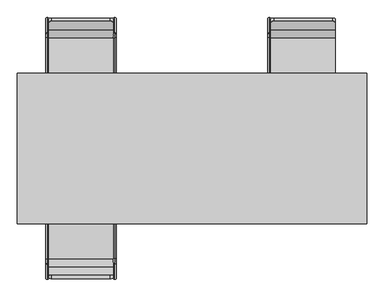
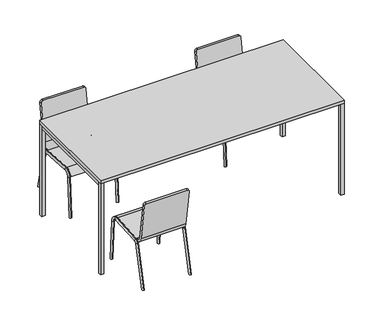
"""IFC4 building model written with IfcOpenShell, lengths in millimetres: furniture geometry."""

from ifc_helpers import new_model, si_unit, point, frame, origin, origin_with_axes, place, context, project, spatial, polyline, circle_curve, ellipse_curve, trimmed, outline, extrude, source, transform, mapped, element, save
from ifc_brep_helpers import plane_surface, cylinder_surface, revolved_surface, advanced_brep


def furniture_b3e58817(model_context):
    return source(origin(), model_context, "Body", "SolidModel", [
        advanced_brep(
        [(10.8556283, 323.0385228, 0.0), (0.8556283, 313.0554101, 0.5809138), (-9.1443717, 323.0385228, 0.0), (0.8556283, 709.1722272, 383.1163586), (0.8556283, 728.5781417, 387.9547965), (0.8556283, 825.3061363, 0.0), (0.8556283, 804.6938637, 0.0), (0.8556283, 333.0554387, 0.0), (0.8556283, 696.6509897, 414.4284246), (0.8556283, 695.489162, 394.4621992), (0.8556283, 397.0871192, 411.8261096), (0.8556283, 398.2489468, 431.792335), (0.8556283, 354.8310131, 374.2173141), (0.8556283, 334.8647877, 375.3791418)],
        [
            (0, 1, circle_curve(frame((0.8556283, 323.0385228, 0.0), z_axis=(0.0, -0.058091383027392335, -0.9983112697039761), x_axis=(0.0, -0.9983112697039761, 0.058091383027392335)), 10.0)),
            (1, 2, circle_curve(frame((0.8556283, 323.0385228, 0.0), z_axis=(0.0, -0.058091383027392335, -0.9983112697039761), x_axis=(0.0, -0.9983112697039761, 0.058091383027392335)), 10.0)),
            (2, 0),
            (3, 4, circle_curve(frame((0.8556283, 718.8751844, 385.5355776), z_axis=(0.0, 0.24192189559966623, -0.9702957262759968), x_axis=(0.0, 0.9702957262759968, 0.24192189559966623)), 10.0)),
            (4, 5),
            (5, 6, ellipse_curve(frame((0.8556283, 815.0, 0.0), z_axis=(0.0, 0.0, 1.0), x_axis=(0.0, 1.0, 0.0)), 10.3061363, 10.0)),
            (6, 3),
            (4, 3, circle_curve(frame((0.8556283, 718.8751844, 385.5355776), z_axis=(0.0, 0.24192189559966623, -0.9702957262759968), x_axis=(0.0, 0.9702957262759968, 0.24192189559966623)), 10.0)),
            (6, 5, ellipse_curve(frame((0.8556283, 815.0, 0.0), z_axis=(0.0, 0.0, 1.0), x_axis=(0.0, 1.0, 0.0)), 10.3061363, 10.0)),
            (2, 7, ellipse_curve(frame((0.8556283, 323.0385228, 0.0), z_axis=(0.0, 0.0, -1.0), x_axis=(0.0, 1.0, 0.0)), 10.0169159, 10.0)),
            (7, 0, ellipse_curve(frame((0.8556283, 323.0385228, 0.0), z_axis=(0.0, 0.0, -1.0), x_axis=(0.0, 1.0, 0.0)), 10.0169159, 10.0)),
            (8, 9, circle_curve(frame((0.8556283, 696.0700758, 404.4453119), z_axis=(0.0, -0.9983112697039764, 0.058091383027386895), x_axis=(0.0, 0.058091383027386895, 0.9983112697039764)), 10.0)),
            (9, 10),
            (10, 11, circle_curve(frame((0.8556283, 397.668033, 421.8092223), z_axis=(0.0, 0.9983112697039764, -0.058091383027386895), x_axis=(0.0, 0.058091383027386895, 0.9983112697039764)), 10.0)),
            (11, 8),
            (9, 8, circle_curve(frame((0.8556283, 696.0700758, 404.4453119), z_axis=(0.0, -0.9983112697039764, 0.058091383027386895), x_axis=(0.0, 0.058091383027386895, 0.9983112697039764)), 10.0)),
            (11, 10, circle_curve(frame((0.8556283, 397.668033, 421.8092223), z_axis=(0.0, 0.9983112697039764, -0.058091383027386895), x_axis=(0.0, 0.058091383027386895, 0.9983112697039764)), 10.0)),
            (10, 12, circle_curve(frame((0.8556283, 394.7634639, 371.8936588), z_axis=(1.0, 0.0, 0.0), x_axis=(0.0, 0.05809138302738633, 0.9983112697039764)), 40.0)),
            (12, 13, circle_curve(frame((0.8556283, 344.8479004, 374.7982279), z_axis=(0.0, 0.058091383027391474, 0.9983112697039761), x_axis=(0.0, -0.9983112697039761, 0.058091383027391474)), 10.0)),
            (13, 11, circle_curve(frame((0.8556283, 394.7634639, 371.8936588), z_axis=(-1.0, 0.0, 0.0), x_axis=(0.0, 0.05809138302738633, 0.9983112697039764)), 60.0)),
            (13, 12, circle_curve(frame((0.8556283, 344.8479004, 374.7982279), z_axis=(0.0, 0.05809138302739081, 0.9983112697039762), x_axis=(0.0, -0.9983112697039762, 0.05809138302739081)), 10.0)),
            (12, 7),
            (1, 13),
            (3, 9, circle_curve(frame((0.8556283, 694.6177913, 379.4875302), z_axis=(1.0, 0.0, 0.0), x_axis=(0.0, 0.9702957262759969, 0.2419218955996659)), 15.0)),
            (8, 4, circle_curve(frame((0.8556283, 694.6177913, 379.4875302), z_axis=(-1.0, 0.0, 0.0), x_axis=(0.0, 0.9702957262759969, 0.2419218955996659)), 35.0)),
        ],
        [
            plane_surface(frame((20.8556283, 323.0385228, 0.0), z_axis=(0.0, -0.058091383027392335, -0.9983112697039761), x_axis=(-1.0, 0.0, 0.0))),
            cylinder_surface(frame((0.8556283, 817.6101503, -10.4687411), z_axis=(0.0, 0.24192189559966623, -0.9702957262759968), x_axis=(0.0, 0.9702957262759968, 0.24192189559966623)), 10.0),
            plane_surface(frame((463.435329, 850.4463822, 0.0), z_axis=(0.0, 0.0, -1.0), x_axis=(-1.0, 0.0, 0.0))),
            cylinder_surface(frame((0.8556283, 696.0700758, 404.4453119), z_axis=(0.0, 0.9983112697039764, -0.058091383027386895), x_axis=(0.0, 0.058091383027386895, 0.9983112697039764)), 10.0),
            revolved_surface(trimmed(ellipse_curve(frame((0.8556283, 397.668033, 421.8092223), z_axis=(0.0, 0.9983112697039764, -0.05809138302738631), x_axis=(0.0, 0.05809138302738631, 0.9983112697039764)), 10.0, 10.0), [point((0.8556283, 397.0871192, 411.8261096))], [point((0.8556283, 398.2489468, 431.792335))], True, "CARTESIAN"), (20.8556283, 394.7634639, 371.8936588), (1.0, 0.0, 0.0)),
            revolved_surface(trimmed(ellipse_curve(frame((0.8556283, 397.668033, 421.8092223), z_axis=(0.0, 0.9983112697039764, -0.05809138302738631), x_axis=(0.0, 0.05809138302738631, 0.9983112697039764)), 10.0, 10.0), [point((0.8556283, 398.2489468, 431.792335))], [point((0.8556283, 397.0871192, 411.8261096))], True, "CARTESIAN"), (20.8556283, 394.7634639, 371.8936588), (1.0, 0.0, 0.0)),
            cylinder_surface(frame((0.8556283, 344.8479004, 374.7982279), z_axis=(0.0, 0.058091383027392335, 0.9983112697039761), x_axis=(0.0, -0.9983112697039761, 0.058091383027392335)), 10.0),
            revolved_surface(trimmed(ellipse_curve(frame((0.8556283, 718.8751844, 385.5355776), z_axis=(0.0, 0.2419218955996659, -0.9702957262759969), x_axis=(0.0, 0.9702957262759969, 0.2419218955996659)), 10.0, 10.0), [point((0.8556283, 709.1722272, 383.1163586))], [point((0.8556283, 728.5781417, 387.9547965))], True, "CARTESIAN"), (20.8556283, 694.6177913, 379.4875302), (1.0, 0.0, 0.0)),
            revolved_surface(trimmed(ellipse_curve(frame((0.8556283, 718.8751844, 385.5355776), z_axis=(0.0, 0.2419218955996659, -0.9702957262759969), x_axis=(0.0, 0.9702957262759969, 0.2419218955996659)), 10.0, 10.0), [point((0.8556283, 728.5781417, 387.9547965))], [point((0.8556283, 709.1722272, 383.1163586))], True, "CARTESIAN"), (20.8556283, 694.6177913, 379.4875302), (1.0, 0.0, 0.0)),
        ],
        [
            (0, [[1, 2, 3]]),
            (1, [[4, 5, 6, 7]]),
            (1, [[8, -7, 9, -5]]),
            (2, [[-3, 10, 11]]),
            (2, [[-6, -9]]),
            (3, [[12, 13, 14, 15]]),
            (3, [[16, -15, 17, -13]]),
            (4, [[-14, 18, 19, 20]]),
            (5, [[-17, -20, 21, -18]]),
            (6, [[-19, 22, -10, -2, 23]]),
            (6, [[-21, -23, -1, -11, -22]]),
            (7, [[-4, 24, -12, 25]]),
            (8, [[-8, -25, -16, -24]]),
        ],
    ),
        advanced_brep(
        [(415.935329, 694.2901891, 414.5657988), (415.935329, 398.2489468, 431.792335), (415.935329, 334.8647877, 375.3791418), (415.935329, 354.8310131, 374.2173141), (415.935329, 397.0871192, 411.8261096), (415.935329, 693.1283614, 394.5995734), (415.935329, 766.4258686, 454.1347035), (415.935329, 817.282073, 794.4215124), (415.935329, 797.5017557, 797.3777006), (415.935329, 746.6455514, 457.0908917), (10.935329, 694.2901891, 414.5657988), (10.935329, 746.6455514, 457.0908917), (10.935329, 797.5017557, 797.3777006), (10.935329, 817.282073, 794.4215124), (10.935329, 766.4258686, 454.1347035), (10.935329, 693.1283614, 394.5995734), (10.935329, 397.0871192, 411.8261096), (10.935329, 354.8310131, 374.2173141), (10.935329, 334.8647877, 375.3791418), (10.935329, 398.2489468, 431.792335), (30.935329, 820.2382612, 814.2018297), (395.935329, 820.2382612, 814.2018297), (30.935329, 800.4579439, 817.1580179), (395.935329, 800.4579439, 817.1580179)],
        [
            (0, 1),
            (1, 2, circle_curve(frame((415.935329, 394.7634639, 371.8936588), z_axis=(1.0, 0.0, 0.0), x_axis=(0.0, 1.0, 0.0)), 60.0)),
            (2, 3),
            (3, 4, circle_curve(frame((415.935329, 394.7634639, 371.8936588), z_axis=(-1.0, 0.0, 0.0), x_axis=(0.0, 1.0, 0.0)), 40.0)),
            (4, 5),
            (5, 6, circle_curve(frame((415.935329, 697.1947582, 464.4813623), z_axis=(1.0, 0.0, 0.0), x_axis=(0.0, 1.0, 0.0)), 70.0)),
            (6, 7),
            (7, 8),
            (8, 9),
            (9, 0, circle_curve(frame((415.935329, 697.1947582, 464.4813623), z_axis=(-1.0, 0.0, 0.0), x_axis=(0.0, 1.0, 0.0)), 50.0)),
            (10, 11, circle_curve(frame((10.935329, 697.1947582, 464.4813623), z_axis=(1.0, 0.0, 0.0), x_axis=(0.0, 1.0, 0.0)), 50.0)),
            (11, 12),
            (12, 13),
            (13, 14),
            (14, 15, circle_curve(frame((10.935329, 697.1947582, 464.4813623), z_axis=(-1.0, 0.0, 0.0), x_axis=(0.0, 1.0, 0.0)), 70.0)),
            (15, 16),
            (16, 17, circle_curve(frame((10.935329, 394.7634639, 371.8936588), z_axis=(1.0, 0.0, 0.0), x_axis=(0.0, 1.0, 0.0)), 40.0)),
            (17, 18),
            (18, 19, circle_curve(frame((10.935329, 394.7634639, 371.8936588), z_axis=(-1.0, 0.0, 0.0), x_axis=(0.0, 1.0, 0.0)), 60.0)),
            (19, 10),
            (0, 10),
            (19, 1),
            (18, 2),
            (17, 3),
            (16, 4),
            (15, 5),
            (14, 6),
            (13, 20, circle_curve(frame((30.935329, 817.282073, 794.4215124), z_axis=(0.0, 0.9890158633619166, -0.14780941112961252), x_axis=(1.0, 0.0, 0.0)), 20.0)),
            (20, 21),
            (21, 7, circle_curve(frame((395.935329, 817.282073, 794.4215124), z_axis=(0.0, 0.9890158633619166, -0.14780941112961252), x_axis=(-1.0, 0.0, 0.0)), 20.0)),
            (20, 22),
            (22, 23),
            (23, 21),
            (11, 9),
            (8, 23, circle_curve(frame((395.935329, 797.5017557, 797.3777006), z_axis=(0.0, -0.9890158633619166, 0.14780941112961252), x_axis=(-1.0, 0.0, 0.0)), 20.0)),
            (22, 12, circle_curve(frame((30.935329, 797.5017557, 797.3777006), z_axis=(0.0, -0.9890158633619166, 0.14780941112961252), x_axis=(1.0, 0.0, 0.0)), 20.0)),
        ],
        [
            plane_surface(frame((415.935329, 400.4940122, 431.6616954), z_axis=(1.0000000000000002, 0.0, 0.0), x_axis=(0.0, -0.9983112697039764, 0.05809138302738736))),
            plane_surface(frame((10.935329, 400.4940122, 431.6616954), z_axis=(-1.0000000000000002, 0.0, 0.0), x_axis=(0.0, 0.9983112697039764, -0.05809138302738736))),
            plane_surface(frame((415.935329, 694.2901891, 414.5657988), z_axis=(0.0, 0.05809138302738736, 0.9983112697039764), x_axis=(-1.0, 0.0, 0.0))),
            cylinder_surface(frame((10.935329, 394.7634639, 371.8936588), z_axis=(1.0, 0.0, 0.0), x_axis=(0.0, 1.0, 0.0)), 60.0),
            plane_surface(frame((415.935329, 334.8647877, 375.3791418), z_axis=(0.0, -0.058091383027390926, -0.9983112697039762), x_axis=(-1.0, 0.0, 0.0))),
            revolved_surface(polyline([(10.935329, 434.7634639, 371.8936588), (415.935329, 434.7634639, 371.8936588)]), (10.935329, 394.7634639, 371.8936588), (-1.0, 0.0, 0.0)),
            plane_surface(frame((415.935329, 397.0871192, 411.8261096), z_axis=(0.0, -0.05809138302738756, -0.9983112697039763), x_axis=(-1.0, 0.0, 0.0))),
            cylinder_surface(frame((10.935329, 697.1947582, 464.4813623), z_axis=(1.0, 0.0, 0.0), x_axis=(0.0, 1.0, 0.0)), 70.0),
            plane_surface(frame((415.935329, 766.4258686, 454.1347035), z_axis=(0.0, 0.9890158633619166, -0.1478094111296125), x_axis=(-1.0, 0.0, 0.0))),
            plane_surface(frame((415.935329, 820.2382612, 814.2018297), z_axis=(0.0, 0.14780941112961524, 0.9890158633619162), x_axis=(-1.0, 0.0, 0.0))),
            plane_surface(frame((415.935329, 800.4579439, 817.1580179), z_axis=(0.0, -0.9890158633619166, 0.14780941112961254), x_axis=(-1.0, 0.0, 0.0))),
            revolved_surface(polyline([(10.935329, 747.1947582, 464.4813623), (415.935329, 747.1947582, 464.4813623)]), (10.935329, 697.1947582, 464.4813623), (-1.0, 0.0, 0.0)),
            cylinder_surface(frame((30.935329, 797.5017557, 797.3777006), z_axis=(0.0, -0.9890158633619166, 0.14780941112961252), x_axis=(1.0, 0.0, 0.0)), 20.0),
            cylinder_surface(frame((395.935329, 797.5017557, 797.3777006), z_axis=(0.0, -0.9890158633619166, 0.14780941112961252), x_axis=(-1.0, 0.0, 0.0)), 20.0),
        ],
        [
            (0, [[1, 2, 3, 4, 5, 6, 7, 8, 9, 10]]),
            (1, [[11, 12, 13, 14, 15, 16, 17, 18, 19, 20]]),
            (2, [[-1, 21, -20, 22]]),
            (3, [[-2, -22, -19, 23]]),
            (4, [[-3, -23, -18, 24]]),
            (5, [[-4, -24, -17, 25]]),
            (6, [[-5, -25, -16, 26]]),
            (7, [[-6, -26, -15, 27]]),
            (8, [[-27, -14, 28, 29, 30, -7]]),
            (9, [[-29, 31, 32, 33]]),
            (10, [[34, -9, 35, -32, 36, -12]]),
            (11, [[-10, -34, -11, -21]]),
            (12, [[-13, -36, -31, -28]]),
            (13, [[-8, -30, -33, -35]]),
        ],
    ),
        advanced_brep(
        [(-973.9849702, -804.6938637, 0.0), (-973.9849702, -825.3061363, 0.0), (-963.9849702, -323.0385228, 0.0), (-973.9849702, -333.0554387, 0.0), (-983.9849702, -323.0385228, 0.0), (-973.9849702, -709.1722272, 383.1163586), (-973.9849702, -728.5781417, 387.9547965), (-973.9849702, -696.6509897, 414.4284246), (-973.9849702, -695.489162, 394.4621992), (-973.9849702, -398.2489468, 431.792335), (-973.9849702, -397.0871192, 411.8261096), (-973.9849702, -334.8647877, 375.3791418), (-973.9849702, -354.8310131, 374.2173141), (-973.9849702, -313.0554101, 0.5809138)],
        [
            (0, 1, ellipse_curve(frame((-973.9849702, -815.0, 0.0), z_axis=(0.0, 0.0, -1.0), x_axis=(0.0, -1.0, 0.0)), 10.3061363, 10.0)),
            (1, 0, ellipse_curve(frame((-973.9849702, -815.0, 0.0), z_axis=(0.0, 0.0, -1.0), x_axis=(0.0, -1.0, 0.0)), 10.3061363, 10.0)),
            (2, 3, ellipse_curve(frame((-973.9849702, -323.0385228, 0.0), z_axis=(0.0, 0.0, -1.0), x_axis=(0.0, -1.0, 0.0)), 10.0169159, 10.0)),
            (3, 4, ellipse_curve(frame((-973.9849702, -323.0385228, 0.0), z_axis=(0.0, 0.0, -1.0), x_axis=(0.0, -1.0, 0.0)), 10.0169159, 10.0)),
            (4, 2),
            (5, 0),
            (1, 6),
            (6, 5, circle_curve(frame((-973.9849702, -718.8751844, 385.5355776), z_axis=(0.0, -0.24192189559966623, -0.9702957262759968), x_axis=(0.0, -0.9702957262759968, 0.24192189559966623)), 10.0)),
            (5, 6, circle_curve(frame((-973.9849702, -718.8751844, 385.5355776), z_axis=(0.0, -0.24192189559966623, -0.9702957262759968), x_axis=(0.0, -0.9702957262759968, 0.24192189559966623)), 10.0)),
            (6, 7, circle_curve(frame((-973.9849702, -694.6177913, 379.4875302), z_axis=(-1.0, 0.0, 0.0), x_axis=(0.0, -0.9702957262759969, 0.2419218955996659)), 35.0)),
            (7, 8, circle_curve(frame((-973.9849702, -696.0700758, 404.4453119), z_axis=(0.0, -0.9983112697039765, -0.05809138302738456), x_axis=(0.0, -0.05809138302738456, 0.9983112697039765)), 10.0)),
            (8, 5, circle_curve(frame((-973.9849702, -694.6177913, 379.4875302), z_axis=(1.0, 0.0, 0.0), x_axis=(0.0, -0.9702957262759969, 0.2419218955996659)), 15.0)),
            (8, 7, circle_curve(frame((-973.9849702, -696.0700758, 404.4453119), z_axis=(0.0, -0.998311269703977, -0.05809138302737549), x_axis=(0.0, -0.05809138302737549, 0.998311269703977)), 10.0)),
            (7, 9),
            (9, 10, circle_curve(frame((-973.9849702, -397.668033, 421.8092223), z_axis=(0.0, -0.9983112697039764, -0.058091383027386895), x_axis=(0.0, -0.058091383027386895, 0.9983112697039764)), 10.0)),
            (10, 8),
            (10, 9, circle_curve(frame((-973.9849702, -397.668033, 421.8092223), z_axis=(0.0, -0.9983112697039764, -0.058091383027386895), x_axis=(0.0, -0.058091383027386895, 0.9983112697039764)), 10.0)),
            (9, 11, circle_curve(frame((-973.9849702, -394.7634639, 371.8936588), z_axis=(-1.0, 0.0, 0.0), x_axis=(0.0, -0.05809138302738633, 0.9983112697039764)), 60.0)),
            (11, 12, circle_curve(frame((-973.9849702, -344.8479004, 374.7982279), z_axis=(0.0, -0.05809138302739081, 0.9983112697039762), x_axis=(0.0, 0.9983112697039762, 0.05809138302739081)), 10.0)),
            (12, 10, circle_curve(frame((-973.9849702, -394.7634639, 371.8936588), z_axis=(1.0, 0.0, 0.0), x_axis=(0.0, -0.05809138302738633, 0.9983112697039764)), 40.0)),
            (12, 11, circle_curve(frame((-973.9849702, -344.8479004, 374.7982279), z_axis=(0.0, -0.05809138302739125, 0.9983112697039761), x_axis=(0.0, 0.9983112697039761, 0.05809138302739125)), 10.0)),
            (4, 13, circle_curve(frame((-973.9849702, -323.0385228, 0.0), z_axis=(0.0, 0.058091383027392335, -0.9983112697039761), x_axis=(0.0, 0.9983112697039761, 0.058091383027392335)), 10.0)),
            (13, 2, circle_curve(frame((-973.9849702, -323.0385228, 0.0), z_axis=(0.0, 0.058091383027392335, -0.9983112697039761), x_axis=(0.0, 0.9983112697039761, 0.058091383027392335)), 10.0)),
            (11, 13),
            (3, 12),
        ],
        [
            plane_surface(frame((-936.564671, -850.4463822, 0.0), z_axis=(0.0, 0.0, -1.0), x_axis=(-1.0, 0.0, 0.0))),
            cylinder_surface(frame((-973.9849702, -817.6101503, -10.4687411), z_axis=(0.0, -0.24192189559966623, -0.9702957262759968), x_axis=(0.0, -0.9702957262759968, 0.24192189559966623)), 10.0),
            revolved_surface(trimmed(ellipse_curve(frame((-973.9849702, -718.8751844, 385.5355776), z_axis=(0.0, 0.2419218955996659, 0.9702957262759969), x_axis=(0.0, -0.9702957262759969, 0.2419218955996659)), 10.0, 10.0), [point((-973.9849702, -709.1722272, 383.1163586))], [point((-973.9849702, -728.5781417, 387.9547965))], True, "CARTESIAN"), (-993.9849702, -694.6177913, 379.4875302), (1.0, 0.0, 0.0)),
            revolved_surface(trimmed(ellipse_curve(frame((-973.9849702, -718.8751844, 385.5355776), z_axis=(0.0, 0.2419218955996659, 0.9702957262759969), x_axis=(0.0, -0.9702957262759969, 0.2419218955996659)), 10.0, 10.0), [point((-973.9849702, -728.5781417, 387.9547965))], [point((-973.9849702, -709.1722272, 383.1163586))], True, "CARTESIAN"), (-993.9849702, -694.6177913, 379.4875302), (1.0, 0.0, 0.0)),
            cylinder_surface(frame((-973.9849702, -696.0700758, 404.4453119), z_axis=(0.0, -0.9983112697039764, -0.058091383027386895), x_axis=(0.0, -0.058091383027386895, 0.9983112697039764)), 10.0),
            revolved_surface(trimmed(ellipse_curve(frame((-973.9849702, -397.668033, 421.8092223), z_axis=(0.0, 0.9983112697039764, 0.05809138302738631), x_axis=(0.0, -0.05809138302738631, 0.9983112697039764)), 10.0, 10.0), [point((-973.9849702, -397.0871192, 411.8261096))], [point((-973.9849702, -398.2489468, 431.792335))], True, "CARTESIAN"), (-993.9849702, -394.7634639, 371.8936588), (1.0, 0.0, 0.0)),
            revolved_surface(trimmed(ellipse_curve(frame((-973.9849702, -397.668033, 421.8092223), z_axis=(0.0, 0.9983112697039764, 0.05809138302738631), x_axis=(0.0, -0.05809138302738631, 0.9983112697039764)), 10.0, 10.0), [point((-973.9849702, -398.2489468, 431.792335))], [point((-973.9849702, -397.0871192, 411.8261096))], True, "CARTESIAN"), (-993.9849702, -394.7634639, 371.8936588), (1.0, 0.0, 0.0)),
            plane_surface(frame((-993.9849702, -323.0385228, 0.0), z_axis=(0.0, 0.058091383027392335, -0.9983112697039761), x_axis=(1.0, 0.0, 0.0))),
            cylinder_surface(frame((-973.9849702, -344.8479004, 374.7982279), z_axis=(0.0, -0.058091383027392335, 0.9983112697039761), x_axis=(0.0, 0.9983112697039761, 0.058091383027392335)), 10.0),
        ],
        [
            (0, [[1, 2]]),
            (0, [[3, 4, 5]]),
            (1, [[6, -2, 7, 8]]),
            (1, [[-7, -1, -6, 9]]),
            (2, [[10, 11, 12, -8]]),
            (3, [[-12, 13, -10, -9]]),
            (4, [[14, 15, 16, -11]]),
            (4, [[-16, 17, -14, -13]]),
            (5, [[18, 19, 20, -15]]),
            (6, [[-20, 21, -18, -17]]),
            (7, [[-5, 22, 23]]),
            (8, [[24, -22, -4, 25, -19]]),
            (8, [[-25, -3, -23, -24, -21]]),
        ],
    ),
        advanced_brep(
        [(-1389.1443717, -323.0385228, 0.0), (-1409.1443717, -323.0385228, 0.0), (-1399.1443717, -313.0554101, 0.5809138), (-1399.1443717, -709.1722272, 383.1163586), (-1399.1443717, -804.6938637, 0.0), (-1399.1443717, -825.3061363, 0.0), (-1399.1443717, -728.5781417, 387.9547965), (-1399.1443717, -333.0554387, 0.0), (-1399.1443717, -696.6509897, 414.4284246), (-1399.1443717, -398.2489468, 431.792335), (-1399.1443717, -397.0871192, 411.8261096), (-1399.1443717, -695.489162, 394.4621992), (-1399.1443717, -334.8647877, 375.3791418), (-1399.1443717, -354.8310131, 374.2173141)],
        [
            (0, 1),
            (1, 2, circle_curve(frame((-1399.1443717, -323.0385228, 0.0), z_axis=(0.0, 0.058091383027392335, -0.9983112697039761), x_axis=(0.0, 0.9983112697039761, 0.058091383027392335)), 10.0)),
            (2, 0, circle_curve(frame((-1399.1443717, -323.0385228, 0.0), z_axis=(0.0, 0.058091383027392335, -0.9983112697039761), x_axis=(0.0, 0.9983112697039761, 0.058091383027392335)), 10.0)),
            (3, 4),
            (4, 5, ellipse_curve(frame((-1399.1443717, -815.0, 0.0), z_axis=(0.0, 0.0, 1.0), x_axis=(0.0, -1.0, 0.0)), 10.3061363, 10.0)),
            (5, 6),
            (6, 3, circle_curve(frame((-1399.1443717, -718.8751844, 385.5355776), z_axis=(0.0, -0.24192189559966623, -0.9702957262759968), x_axis=(0.0, -0.9702957262759968, 0.24192189559966623)), 10.0)),
            (5, 4, ellipse_curve(frame((-1399.1443717, -815.0, 0.0), z_axis=(0.0, 0.0, 1.0), x_axis=(0.0, -1.0, 0.0)), 10.3061363, 10.0)),
            (3, 6, circle_curve(frame((-1399.1443717, -718.8751844, 385.5355776), z_axis=(0.0, -0.24192189559966623, -0.9702957262759968), x_axis=(0.0, -0.9702957262759968, 0.24192189559966623)), 10.0)),
            (0, 7, ellipse_curve(frame((-1399.1443717, -323.0385228, 0.0), z_axis=(0.0, 0.0, -1.0), x_axis=(0.0, -1.0, 0.0)), 10.0169159, 10.0)),
            (7, 1, ellipse_curve(frame((-1399.1443717, -323.0385228, 0.0), z_axis=(0.0, 0.0, -1.0), x_axis=(0.0, -1.0, 0.0)), 10.0169159, 10.0)),
            (8, 9),
            (9, 10, circle_curve(frame((-1399.1443717, -397.668033, 421.8092223), z_axis=(0.0, -0.9983112697039764, -0.058091383027386895), x_axis=(0.0, -0.058091383027386895, 0.9983112697039764)), 10.0)),
            (10, 11),
            (11, 8, circle_curve(frame((-1399.1443717, -696.0700758, 404.4453119), z_axis=(0.0, 0.9983112697039764, 0.058091383027386895), x_axis=(0.0, -0.058091383027386895, 0.9983112697039764)), 10.0)),
            (10, 9, circle_curve(frame((-1399.1443717, -397.668033, 421.8092223), z_axis=(0.0, -0.9983112697039764, -0.058091383027386895), x_axis=(0.0, -0.058091383027386895, 0.9983112697039764)), 10.0)),
            (8, 11, circle_curve(frame((-1399.1443717, -696.0700758, 404.4453119), z_axis=(0.0, 0.9983112697039764, 0.058091383027386895), x_axis=(0.0, -0.058091383027386895, 0.9983112697039764)), 10.0)),
            (9, 12, circle_curve(frame((-1399.1443717, -394.7634639, 371.8936588), z_axis=(-1.0, 0.0, 0.0), x_axis=(0.0, -0.05809138302738633, 0.9983112697039764)), 60.0)),
            (12, 13, circle_curve(frame((-1399.1443717, -344.8479004, 374.7982279), z_axis=(0.0, -0.058091383027391474, 0.9983112697039761), x_axis=(0.0, 0.9983112697039761, 0.058091383027391474)), 10.0)),
            (13, 10, circle_curve(frame((-1399.1443717, -394.7634639, 371.8936588), z_axis=(1.0, 0.0, 0.0), x_axis=(0.0, -0.05809138302738633, 0.9983112697039764)), 40.0)),
            (13, 12, circle_curve(frame((-1399.1443717, -344.8479004, 374.7982279), z_axis=(0.0, -0.05809138302739081, 0.9983112697039762), x_axis=(0.0, 0.9983112697039762, 0.05809138302739081)), 10.0)),
            (12, 2),
            (7, 13),
            (6, 8, circle_curve(frame((-1399.1443717, -694.6177913, 379.4875302), z_axis=(-1.0, 0.0, 0.0), x_axis=(0.0, -0.9702957262759969, 0.2419218955996659)), 35.0)),
            (11, 3, circle_curve(frame((-1399.1443717, -694.6177913, 379.4875302), z_axis=(1.0, 0.0, 0.0), x_axis=(0.0, -0.9702957262759969, 0.2419218955996659)), 15.0)),
        ],
        [
            plane_surface(frame((-1379.1443717, -323.0385228, 0.0), z_axis=(0.0, 0.058091383027392335, -0.9983112697039761), x_axis=(-1.0, 0.0, 0.0))),
            cylinder_surface(frame((-1399.1443717, -817.6101503, -10.4687411), z_axis=(0.0, -0.24192189559966623, -0.9702957262759968), x_axis=(0.0, -0.9702957262759968, 0.24192189559966623)), 10.0),
            plane_surface(frame((-936.564671, -850.4463822, 0.0), z_axis=(0.0, 0.0, -1.0), x_axis=(-1.0, 0.0, 0.0))),
            cylinder_surface(frame((-1399.1443717, -696.0700758, 404.4453119), z_axis=(0.0, -0.9983112697039764, -0.058091383027386895), x_axis=(0.0, -0.058091383027386895, 0.9983112697039764)), 10.0),
            revolved_surface(trimmed(ellipse_curve(frame((-1399.1443717, -397.668033, 421.8092223), z_axis=(0.0, 0.9983112697039764, 0.05809138302738631), x_axis=(0.0, -0.05809138302738631, 0.9983112697039764)), 10.0, 10.0), [point((-1399.1443717, -397.0871192, 411.8261096))], [point((-1399.1443717, -398.2489468, 431.792335))], True, "CARTESIAN"), (-1379.1443717, -394.7634639, 371.8936588), (1.0, 0.0, 0.0)),
            revolved_surface(trimmed(ellipse_curve(frame((-1399.1443717, -397.668033, 421.8092223), z_axis=(0.0, 0.9983112697039764, 0.05809138302738631), x_axis=(0.0, -0.05809138302738631, 0.9983112697039764)), 10.0, 10.0), [point((-1399.1443717, -398.2489468, 431.792335))], [point((-1399.1443717, -397.0871192, 411.8261096))], True, "CARTESIAN"), (-1379.1443717, -394.7634639, 371.8936588), (1.0, 0.0, 0.0)),
            cylinder_surface(frame((-1399.1443717, -344.8479004, 374.7982279), z_axis=(0.0, -0.058091383027392335, 0.9983112697039761), x_axis=(0.0, 0.9983112697039761, 0.058091383027392335)), 10.0),
            revolved_surface(trimmed(ellipse_curve(frame((-1399.1443717, -718.8751844, 385.5355776), z_axis=(0.0, 0.2419218955996659, 0.9702957262759969), x_axis=(0.0, -0.9702957262759969, 0.2419218955996659)), 10.0, 10.0), [point((-1399.1443717, -709.1722272, 383.1163586))], [point((-1399.1443717, -728.5781417, 387.9547965))], True, "CARTESIAN"), (-1379.1443717, -694.6177913, 379.4875302), (1.0, 0.0, 0.0)),
            revolved_surface(trimmed(ellipse_curve(frame((-1399.1443717, -718.8751844, 385.5355776), z_axis=(0.0, 0.2419218955996659, 0.9702957262759969), x_axis=(0.0, -0.9702957262759969, 0.2419218955996659)), 10.0, 10.0), [point((-1399.1443717, -728.5781417, 387.9547965))], [point((-1399.1443717, -709.1722272, 383.1163586))], True, "CARTESIAN"), (-1379.1443717, -694.6177913, 379.4875302), (1.0, 0.0, 0.0)),
        ],
        [
            (0, [[1, 2, 3]]),
            (1, [[4, 5, 6, 7]]),
            (1, [[-6, 8, -4, 9]]),
            (2, [[-8, -5]]),
            (2, [[10, 11, -1]]),
            (3, [[12, 13, 14, 15]]),
            (3, [[-14, 16, -12, 17]]),
            (4, [[18, 19, 20, -13]]),
            (5, [[-20, 21, -18, -16]]),
            (6, [[22, -2, -11, 23, -19]]),
            (6, [[-23, -10, -3, -22, -21]]),
            (7, [[24, -15, 25, -7]]),
            (8, [[-25, -17, -24, -9]]),
        ],
    ),
        advanced_brep(
        [(-984.064671, -694.2901891, 414.5657988), (-984.064671, -746.6455514, 457.0908917), (-984.064671, -797.5017557, 797.3777006), (-984.064671, -817.282073, 794.4215124), (-984.064671, -766.4258686, 454.1347035), (-984.064671, -693.1283614, 394.5995734), (-984.064671, -397.0871192, 411.8261096), (-984.064671, -354.8310131, 374.2173141), (-984.064671, -334.8647877, 375.3791418), (-984.064671, -398.2489468, 431.792335), (-1389.064671, -694.2901891, 414.5657988), (-1389.064671, -398.2489468, 431.792335), (-1389.064671, -334.8647877, 375.3791418), (-1389.064671, -354.8310131, 374.2173141), (-1389.064671, -397.0871192, 411.8261096), (-1389.064671, -693.1283614, 394.5995734), (-1389.064671, -766.4258686, 454.1347035), (-1389.064671, -817.282073, 794.4215124), (-1389.064671, -797.5017557, 797.3777006), (-1389.064671, -746.6455514, 457.0908917), (-1004.064671, -820.2382612, 814.2018297), (-1369.064671, -820.2382612, 814.2018297), (-1004.064671, -800.4579439, 817.1580179), (-1369.064671, -800.4579439, 817.1580179)],
        [
            (0, 1, circle_curve(frame((-984.064671, -697.1947582, 464.4813623), z_axis=(-1.0, 0.0, 0.0), x_axis=(0.0, -1.0, 0.0)), 50.0)),
            (1, 2),
            (2, 3),
            (3, 4),
            (4, 5, circle_curve(frame((-984.064671, -697.1947582, 464.4813623), z_axis=(1.0, 0.0, 0.0), x_axis=(0.0, -1.0, 0.0)), 70.0)),
            (5, 6),
            (6, 7, circle_curve(frame((-984.064671, -394.7634639, 371.8936588), z_axis=(-1.0, 0.0, 0.0), x_axis=(0.0, -1.0, 0.0)), 40.0)),
            (7, 8),
            (8, 9, circle_curve(frame((-984.064671, -394.7634639, 371.8936588), z_axis=(1.0, 0.0, 0.0), x_axis=(0.0, -1.0, 0.0)), 60.0)),
            (9, 0),
            (10, 11),
            (11, 12, circle_curve(frame((-1389.064671, -394.7634639, 371.8936588), z_axis=(-1.0, 0.0, 0.0), x_axis=(0.0, -1.0, 0.0)), 60.0)),
            (12, 13),
            (13, 14, circle_curve(frame((-1389.064671, -394.7634639, 371.8936588), z_axis=(1.0, 0.0, 0.0), x_axis=(0.0, -1.0, 0.0)), 40.0)),
            (14, 15),
            (15, 16, circle_curve(frame((-1389.064671, -697.1947582, 464.4813623), z_axis=(-1.0, 0.0, 0.0), x_axis=(0.0, -1.0, 0.0)), 70.0)),
            (16, 17),
            (17, 18),
            (18, 19),
            (19, 10, circle_curve(frame((-1389.064671, -697.1947582, 464.4813623), z_axis=(1.0, 0.0, 0.0), x_axis=(0.0, -1.0, 0.0)), 50.0)),
            (9, 11),
            (10, 0),
            (8, 12),
            (7, 13),
            (6, 14),
            (5, 15),
            (4, 16),
            (3, 20, circle_curve(frame((-1004.064671, -817.282073, 794.4215124), z_axis=(0.0, -0.9890158633619166, -0.14780941112961252), x_axis=(-1.0, 0.0, 0.0)), 20.0)),
            (20, 21),
            (21, 17, circle_curve(frame((-1369.064671, -817.282073, 794.4215124), z_axis=(0.0, -0.9890158633619166, -0.14780941112961252), x_axis=(1.0, 0.0, 0.0)), 20.0)),
            (20, 22),
            (22, 23),
            (23, 21),
            (18, 23, circle_curve(frame((-1369.064671, -797.5017557, 797.3777006), z_axis=(0.0, 0.9890158633619166, 0.14780941112961252), x_axis=(1.0, 0.0, 0.0)), 20.0)),
            (22, 2, circle_curve(frame((-1004.064671, -797.5017557, 797.3777006), z_axis=(0.0, 0.9890158633619166, 0.14780941112961252), x_axis=(-1.0, 0.0, 0.0)), 20.0)),
            (1, 19),
        ],
        [
            plane_surface(frame((-984.064671, -400.4940122, 431.6616954), z_axis=(1.0000000000000002, 0.0, 0.0), x_axis=(0.0, 0.9983112697039764, 0.05809138302738736))),
            plane_surface(frame((-1389.064671, -400.4940122, 431.6616954), z_axis=(-1.0000000000000002, 0.0, 0.0), x_axis=(0.0, -0.9983112697039764, -0.05809138302738736))),
            plane_surface(frame((-984.064671, -694.2901891, 414.5657988), z_axis=(0.0, -0.05809138302738736, 0.9983112697039764), x_axis=(-1.0, 0.0, 0.0))),
            cylinder_surface(frame((-1389.064671, -394.7634639, 371.8936588), z_axis=(1.0, 0.0, 0.0), x_axis=(0.0, -1.0, 0.0)), 60.0),
            plane_surface(frame((-984.064671, -334.8647877, 375.3791418), z_axis=(0.0, 0.058091383027390926, -0.9983112697039762), x_axis=(-1.0, 0.0, 0.0))),
            revolved_surface(polyline([(-1389.064671, -434.7634639, 371.8936588), (-984.064671, -434.7634639, 371.8936588)]), (-1389.064671, -394.7634639, 371.8936588), (-1.0, 0.0, 0.0)),
            plane_surface(frame((-984.064671, -397.0871192, 411.8261096), z_axis=(0.0, 0.05809138302738756, -0.9983112697039763), x_axis=(-1.0, 0.0, 0.0))),
            cylinder_surface(frame((-1389.064671, -697.1947582, 464.4813623), z_axis=(1.0, 0.0, 0.0), x_axis=(0.0, -1.0, 0.0)), 70.0),
            plane_surface(frame((-984.064671, -766.4258686, 454.1347035), z_axis=(0.0, -0.9890158633619166, -0.1478094111296125), x_axis=(-1.0, 0.0, 0.0))),
            plane_surface(frame((-984.064671, -820.2382612, 814.2018297), z_axis=(0.0, -0.14780941112961524, 0.9890158633619162), x_axis=(-1.0, 0.0, 0.0))),
            plane_surface(frame((-984.064671, -800.4579439, 817.1580179), z_axis=(0.0, 0.9890158633619166, 0.14780941112961254), x_axis=(-1.0, 0.0, 0.0))),
            revolved_surface(polyline([(-1389.064671, -747.1947582, 464.4813623), (-984.064671, -747.1947582, 464.4813623)]), (-1389.064671, -697.1947582, 464.4813623), (-1.0, 0.0, 0.0)),
            cylinder_surface(frame((-1369.064671, -797.5017557, 797.3777006), z_axis=(0.0, 0.9890158633619166, 0.14780941112961252), x_axis=(1.0, 0.0, 0.0)), 20.0),
            cylinder_surface(frame((-1004.064671, -797.5017557, 797.3777006), z_axis=(0.0, 0.9890158633619166, 0.14780941112961252), x_axis=(-1.0, 0.0, 0.0)), 20.0),
        ],
        [
            (0, [[1, 2, 3, 4, 5, 6, 7, 8, 9, 10]]),
            (1, [[11, 12, 13, 14, 15, 16, 17, 18, 19, 20]]),
            (2, [[21, -11, 22, -10]]),
            (3, [[23, -12, -21, -9]]),
            (4, [[24, -13, -23, -8]]),
            (5, [[25, -14, -24, -7]]),
            (6, [[26, -15, -25, -6]]),
            (7, [[27, -16, -26, -5]]),
            (8, [[-4, 28, 29, 30, -17, -27]]),
            (9, [[31, 32, 33, -29]]),
            (10, [[-19, 34, -32, 35, -2, 36]]),
            (11, [[-22, -20, -36, -1]]),
            (12, [[-30, -33, -34, -18]]),
            (13, [[-35, -31, -28, -3]]),
        ],
    ),
        advanced_brep(
        [(-973.9849702, 804.6938637, 0.0), (-973.9849702, 825.3061363, 0.0), (-963.9849702, 323.0385228, 0.0), (-983.9849702, 323.0385228, 0.0), (-973.9849702, 333.0554387, 0.0), (-973.9849702, 709.1722272, 383.1163586), (-973.9849702, 728.5781417, 387.9547965), (-973.9849702, 695.489162, 394.4621992), (-973.9849702, 696.6509897, 414.4284246), (-973.9849702, 397.0871192, 411.8261096), (-973.9849702, 398.2489468, 431.792335), (-973.9849702, 354.8310131, 374.2173141), (-973.9849702, 334.8647877, 375.3791418), (-973.9849702, 313.0554101, 0.5809138)],
        [
            (0, 1, ellipse_curve(frame((-973.9849702, 815.0, 0.0), z_axis=(0.0, 0.0, -1.0), x_axis=(0.0, 1.0, 0.0)), 10.3061363, 10.0)),
            (1, 0, ellipse_curve(frame((-973.9849702, 815.0, 0.0), z_axis=(0.0, 0.0, -1.0), x_axis=(0.0, 1.0, 0.0)), 10.3061363, 10.0)),
            (2, 3),
            (3, 4, ellipse_curve(frame((-973.9849702, 323.0385228, 0.0), z_axis=(0.0, 0.0, -1.0), x_axis=(0.0, 1.0, 0.0)), 10.0169159, 10.0)),
            (4, 2, ellipse_curve(frame((-973.9849702, 323.0385228, 0.0), z_axis=(0.0, 0.0, -1.0), x_axis=(0.0, 1.0, 0.0)), 10.0169159, 10.0)),
            (5, 6, circle_curve(frame((-973.9849702, 718.8751844, 385.5355776), z_axis=(0.0, 0.24192189559966623, -0.9702957262759968), x_axis=(0.0, 0.9702957262759968, 0.24192189559966623)), 10.0)),
            (6, 1),
            (0, 5),
            (6, 5, circle_curve(frame((-973.9849702, 718.8751844, 385.5355776), z_axis=(0.0, 0.24192189559966623, -0.9702957262759968), x_axis=(0.0, 0.9702957262759968, 0.24192189559966623)), 10.0)),
            (5, 7, circle_curve(frame((-973.9849702, 694.6177913, 379.4875302), z_axis=(1.0, 0.0, 0.0), x_axis=(0.0, 0.9702957262759969, 0.2419218955996659)), 15.0)),
            (7, 8, circle_curve(frame((-973.9849702, 696.0700758, 404.4453119), z_axis=(0.0, 0.998311269703977, -0.058091383027376764), x_axis=(0.0, 0.058091383027376764, 0.998311269703977)), 10.0)),
            (8, 6, circle_curve(frame((-973.9849702, 694.6177913, 379.4875302), z_axis=(-1.0, 0.0, 0.0), x_axis=(0.0, 0.9702957262759969, 0.2419218955996659)), 35.0)),
            (8, 7, circle_curve(frame((-973.9849702, 696.0700758, 404.4453119), z_axis=(0.0, 0.9983112697039765, -0.05809138302738498), x_axis=(0.0, 0.05809138302738498, 0.9983112697039765)), 10.0)),
            (7, 9),
            (9, 10, circle_curve(frame((-973.9849702, 397.668033, 421.8092223), z_axis=(0.0, 0.9983112697039764, -0.058091383027386895), x_axis=(0.0, 0.058091383027386895, 0.9983112697039764)), 10.0)),
            (10, 8),
            (10, 9, circle_curve(frame((-973.9849702, 397.668033, 421.8092223), z_axis=(0.0, 0.9983112697039764, -0.058091383027386895), x_axis=(0.0, 0.058091383027386895, 0.9983112697039764)), 10.0)),
            (9, 11, circle_curve(frame((-973.9849702, 394.7634639, 371.8936588), z_axis=(1.0, 0.0, 0.0), x_axis=(0.0, 0.05809138302738633, 0.9983112697039764)), 40.0)),
            (11, 12, circle_curve(frame((-973.9849702, 344.8479004, 374.7982279), z_axis=(0.0, 0.058091383027391474, 0.9983112697039761), x_axis=(0.0, -0.9983112697039761, 0.058091383027391474)), 10.0)),
            (12, 10, circle_curve(frame((-973.9849702, 394.7634639, 371.8936588), z_axis=(-1.0, 0.0, 0.0), x_axis=(0.0, 0.05809138302738633, 0.9983112697039764)), 60.0)),
            (12, 11, circle_curve(frame((-973.9849702, 344.8479004, 374.7982279), z_axis=(0.0, 0.05809138302739081, 0.9983112697039762), x_axis=(0.0, -0.9983112697039762, 0.05809138302739081)), 10.0)),
            (2, 13, circle_curve(frame((-973.9849702, 323.0385228, 0.0), z_axis=(0.0, -0.058091383027392335, -0.9983112697039761), x_axis=(0.0, -0.9983112697039761, 0.058091383027392335)), 10.0)),
            (13, 3, circle_curve(frame((-973.9849702, 323.0385228, 0.0), z_axis=(0.0, -0.058091383027392335, -0.9983112697039761), x_axis=(0.0, -0.9983112697039761, 0.058091383027392335)), 10.0)),
            (11, 4),
            (13, 12),
        ],
        [
            plane_surface(frame((-936.564671, 850.4463822, 0.0), z_axis=(0.0, 0.0, -1.0), x_axis=(-1.0, 0.0, 0.0))),
            cylinder_surface(frame((-973.9849702, 817.6101503, -10.4687411), z_axis=(0.0, 0.24192189559966623, -0.9702957262759968), x_axis=(0.0, 0.9702957262759968, 0.24192189559966623)), 10.0),
            revolved_surface(trimmed(ellipse_curve(frame((-973.9849702, 718.8751844, 385.5355776), z_axis=(0.0, 0.2419218955996659, -0.9702957262759969), x_axis=(0.0, 0.9702957262759969, 0.2419218955996659)), 10.0, 10.0), [point((-973.9849702, 709.1722272, 383.1163586))], [point((-973.9849702, 728.5781417, 387.9547965))], True, "CARTESIAN"), (-993.9849702, 694.6177913, 379.4875302), (1.0, 0.0, 0.0)),
            revolved_surface(trimmed(ellipse_curve(frame((-973.9849702, 718.8751844, 385.5355776), z_axis=(0.0, 0.2419218955996659, -0.9702957262759969), x_axis=(0.0, 0.9702957262759969, 0.2419218955996659)), 10.0, 10.0), [point((-973.9849702, 728.5781417, 387.9547965))], [point((-973.9849702, 709.1722272, 383.1163586))], True, "CARTESIAN"), (-993.9849702, 694.6177913, 379.4875302), (1.0, 0.0, 0.0)),
            cylinder_surface(frame((-973.9849702, 696.0700758, 404.4453119), z_axis=(0.0, 0.9983112697039764, -0.058091383027386895), x_axis=(0.0, 0.058091383027386895, 0.9983112697039764)), 10.0),
            revolved_surface(trimmed(ellipse_curve(frame((-973.9849702, 397.668033, 421.8092223), z_axis=(0.0, 0.9983112697039764, -0.05809138302738631), x_axis=(0.0, 0.05809138302738631, 0.9983112697039764)), 10.0, 10.0), [point((-973.9849702, 397.0871192, 411.8261096))], [point((-973.9849702, 398.2489468, 431.792335))], True, "CARTESIAN"), (-993.9849702, 394.7634639, 371.8936588), (1.0, 0.0, 0.0)),
            revolved_surface(trimmed(ellipse_curve(frame((-973.9849702, 397.668033, 421.8092223), z_axis=(0.0, 0.9983112697039764, -0.05809138302738631), x_axis=(0.0, 0.05809138302738631, 0.9983112697039764)), 10.0, 10.0), [point((-973.9849702, 398.2489468, 431.792335))], [point((-973.9849702, 397.0871192, 411.8261096))], True, "CARTESIAN"), (-993.9849702, 394.7634639, 371.8936588), (1.0, 0.0, 0.0)),
            plane_surface(frame((-993.9849702, 323.0385228, 0.0), z_axis=(0.0, -0.058091383027392335, -0.9983112697039761), x_axis=(1.0, 0.0, 0.0))),
            cylinder_surface(frame((-973.9849702, 344.8479004, 374.7982279), z_axis=(0.0, 0.058091383027392335, 0.9983112697039761), x_axis=(0.0, -0.9983112697039761, 0.058091383027392335)), 10.0),
        ],
        [
            (0, [[1, 2]]),
            (0, [[3, 4, 5]]),
            (1, [[6, 7, -1, 8]]),
            (1, [[9, -8, -2, -7]]),
            (2, [[-6, 10, 11, 12]]),
            (3, [[-9, -12, 13, -10]]),
            (4, [[-11, 14, 15, 16]]),
            (4, [[-13, -16, 17, -14]]),
            (5, [[-15, 18, 19, 20]]),
            (6, [[-17, -20, 21, -18]]),
            (7, [[22, 23, -3]]),
            (8, [[-19, 24, -4, -23, 25]]),
            (8, [[-21, -25, -22, -5, -24]]),
        ],
    ),
        advanced_brep(
        [(-1389.1443717, 323.0385228, 0.0), (-1399.1443717, 313.0554101, 0.5809138), (-1409.1443717, 323.0385228, 0.0), (-1399.1443717, 709.1722272, 383.1163586), (-1399.1443717, 728.5781417, 387.9547965), (-1399.1443717, 825.3061363, 0.0), (-1399.1443717, 804.6938637, 0.0), (-1399.1443717, 333.0554387, 0.0), (-1399.1443717, 696.6509897, 414.4284246), (-1399.1443717, 695.489162, 394.4621992), (-1399.1443717, 397.0871192, 411.8261096), (-1399.1443717, 398.2489468, 431.792335), (-1399.1443717, 354.8310131, 374.2173141), (-1399.1443717, 334.8647877, 375.3791418)],
        [
            (0, 1, circle_curve(frame((-1399.1443717, 323.0385228, 0.0), z_axis=(0.0, -0.058091383027392335, -0.9983112697039761), x_axis=(0.0, -0.9983112697039761, 0.058091383027392335)), 10.0)),
            (1, 2, circle_curve(frame((-1399.1443717, 323.0385228, 0.0), z_axis=(0.0, -0.058091383027392335, -0.9983112697039761), x_axis=(0.0, -0.9983112697039761, 0.058091383027392335)), 10.0)),
            (2, 0),
            (3, 4, circle_curve(frame((-1399.1443717, 718.8751844, 385.5355776), z_axis=(0.0, 0.24192189559966623, -0.9702957262759968), x_axis=(0.0, 0.9702957262759968, 0.24192189559966623)), 10.0)),
            (4, 5),
            (5, 6, ellipse_curve(frame((-1399.1443717, 815.0, 0.0), z_axis=(0.0, 0.0, 1.0), x_axis=(0.0, 1.0, 0.0)), 10.3061363, 10.0)),
            (6, 3),
            (4, 3, circle_curve(frame((-1399.1443717, 718.8751844, 385.5355776), z_axis=(0.0, 0.24192189559966623, -0.9702957262759968), x_axis=(0.0, 0.9702957262759968, 0.24192189559966623)), 10.0)),
            (6, 5, ellipse_curve(frame((-1399.1443717, 815.0, 0.0), z_axis=(0.0, 0.0, 1.0), x_axis=(0.0, 1.0, 0.0)), 10.3061363, 10.0)),
            (2, 7, ellipse_curve(frame((-1399.1443717, 323.0385228, 0.0), z_axis=(0.0, 0.0, -1.0), x_axis=(0.0, 1.0, 0.0)), 10.0169159, 10.0)),
            (7, 0, ellipse_curve(frame((-1399.1443717, 323.0385228, 0.0), z_axis=(0.0, 0.0, -1.0), x_axis=(0.0, 1.0, 0.0)), 10.0169159, 10.0)),
            (8, 9, circle_curve(frame((-1399.1443717, 696.0700758, 404.4453119), z_axis=(0.0, -0.9983112697039764, 0.058091383027386895), x_axis=(0.0, 0.058091383027386895, 0.9983112697039764)), 10.0)),
            (9, 10),
            (10, 11, circle_curve(frame((-1399.1443717, 397.668033, 421.8092223), z_axis=(0.0, 0.9983112697039764, -0.058091383027386895), x_axis=(0.0, 0.058091383027386895, 0.9983112697039764)), 10.0)),
            (11, 8),
            (9, 8, circle_curve(frame((-1399.1443717, 696.0700758, 404.4453119), z_axis=(0.0, -0.9983112697039764, 0.058091383027386895), x_axis=(0.0, 0.058091383027386895, 0.9983112697039764)), 10.0)),
            (11, 10, circle_curve(frame((-1399.1443717, 397.668033, 421.8092223), z_axis=(0.0, 0.9983112697039764, -0.058091383027386895), x_axis=(0.0, 0.058091383027386895, 0.9983112697039764)), 10.0)),
            (10, 12, circle_curve(frame((-1399.1443717, 394.7634639, 371.8936588), z_axis=(1.0, 0.0, 0.0), x_axis=(0.0, 0.05809138302738633, 0.9983112697039764)), 40.0)),
            (12, 13, circle_curve(frame((-1399.1443717, 344.8479004, 374.7982279), z_axis=(0.0, 0.058091383027391474, 0.9983112697039761), x_axis=(0.0, -0.9983112697039761, 0.058091383027391474)), 10.0)),
            (13, 11, circle_curve(frame((-1399.1443717, 394.7634639, 371.8936588), z_axis=(-1.0, 0.0, 0.0), x_axis=(0.0, 0.05809138302738633, 0.9983112697039764)), 60.0)),
            (13, 12, circle_curve(frame((-1399.1443717, 344.8479004, 374.7982279), z_axis=(0.0, 0.05809138302739081, 0.9983112697039762), x_axis=(0.0, -0.9983112697039762, 0.05809138302739081)), 10.0)),
            (12, 7),
            (1, 13),
            (3, 9, circle_curve(frame((-1399.1443717, 694.6177913, 379.4875302), z_axis=(1.0, 0.0, 0.0), x_axis=(0.0, 0.9702957262759969, 0.2419218955996659)), 15.0)),
            (8, 4, circle_curve(frame((-1399.1443717, 694.6177913, 379.4875302), z_axis=(-1.0, 0.0, 0.0), x_axis=(0.0, 0.9702957262759969, 0.2419218955996659)), 35.0)),
        ],
        [
            plane_surface(frame((-1379.1443717, 323.0385228, 0.0), z_axis=(0.0, -0.058091383027392335, -0.9983112697039761), x_axis=(-1.0, 0.0, 0.0))),
            cylinder_surface(frame((-1399.1443717, 817.6101503, -10.4687411), z_axis=(0.0, 0.24192189559966623, -0.9702957262759968), x_axis=(0.0, 0.9702957262759968, 0.24192189559966623)), 10.0),
            plane_surface(frame((-936.564671, 850.4463822, 0.0), z_axis=(0.0, 0.0, -1.0), x_axis=(-1.0, 0.0, 0.0))),
            cylinder_surface(frame((-1399.1443717, 696.0700758, 404.4453119), z_axis=(0.0, 0.9983112697039764, -0.058091383027386895), x_axis=(0.0, 0.058091383027386895, 0.9983112697039764)), 10.0),
            revolved_surface(trimmed(ellipse_curve(frame((-1399.1443717, 397.668033, 421.8092223), z_axis=(0.0, 0.9983112697039764, -0.05809138302738631), x_axis=(0.0, 0.05809138302738631, 0.9983112697039764)), 10.0, 10.0), [point((-1399.1443717, 397.0871192, 411.8261096))], [point((-1399.1443717, 398.2489468, 431.792335))], True, "CARTESIAN"), (-1379.1443717, 394.7634639, 371.8936588), (1.0, 0.0, 0.0)),
            revolved_surface(trimmed(ellipse_curve(frame((-1399.1443717, 397.668033, 421.8092223), z_axis=(0.0, 0.9983112697039764, -0.05809138302738631), x_axis=(0.0, 0.05809138302738631, 0.9983112697039764)), 10.0, 10.0), [point((-1399.1443717, 398.2489468, 431.792335))], [point((-1399.1443717, 397.0871192, 411.8261096))], True, "CARTESIAN"), (-1379.1443717, 394.7634639, 371.8936588), (1.0, 0.0, 0.0)),
            cylinder_surface(frame((-1399.1443717, 344.8479004, 374.7982279), z_axis=(0.0, 0.058091383027392335, 0.9983112697039761), x_axis=(0.0, -0.9983112697039761, 0.058091383027392335)), 10.0),
            revolved_surface(trimmed(ellipse_curve(frame((-1399.1443717, 718.8751844, 385.5355776), z_axis=(0.0, 0.2419218955996659, -0.9702957262759969), x_axis=(0.0, 0.9702957262759969, 0.2419218955996659)), 10.0, 10.0), [point((-1399.1443717, 709.1722272, 383.1163586))], [point((-1399.1443717, 728.5781417, 387.9547965))], True, "CARTESIAN"), (-1379.1443717, 694.6177913, 379.4875302), (1.0, 0.0, 0.0)),
            revolved_surface(trimmed(ellipse_curve(frame((-1399.1443717, 718.8751844, 385.5355776), z_axis=(0.0, 0.2419218955996659, -0.9702957262759969), x_axis=(0.0, 0.9702957262759969, 0.2419218955996659)), 10.0, 10.0), [point((-1399.1443717, 728.5781417, 387.9547965))], [point((-1399.1443717, 709.1722272, 383.1163586))], True, "CARTESIAN"), (-1379.1443717, 694.6177913, 379.4875302), (1.0, 0.0, 0.0)),
        ],
        [
            (0, [[1, 2, 3]]),
            (1, [[4, 5, 6, 7]]),
            (1, [[8, -7, 9, -5]]),
            (2, [[-3, 10, 11]]),
            (2, [[-6, -9]]),
            (3, [[12, 13, 14, 15]]),
            (3, [[16, -15, 17, -13]]),
            (4, [[-14, 18, 19, 20]]),
            (5, [[-17, -20, 21, -18]]),
            (6, [[-19, 22, -10, -2, 23]]),
            (6, [[-21, -23, -1, -11, -22]]),
            (7, [[-4, 24, -12, 25]]),
            (8, [[-8, -25, -16, -24]]),
        ],
    ),
        advanced_brep(
        [(-984.064671, 694.2901891, 414.5657988), (-984.064671, 398.2489468, 431.792335), (-984.064671, 334.8647877, 375.3791418), (-984.064671, 354.8310131, 374.2173141), (-984.064671, 397.0871192, 411.8261096), (-984.064671, 693.1283614, 394.5995734), (-984.064671, 766.4258686, 454.1347035), (-984.064671, 817.282073, 794.4215124), (-984.064671, 797.5017557, 797.3777006), (-984.064671, 746.6455514, 457.0908917), (-1389.064671, 694.2901891, 414.5657988), (-1389.064671, 746.6455514, 457.0908917), (-1389.064671, 797.5017557, 797.3777006), (-1389.064671, 817.282073, 794.4215124), (-1389.064671, 766.4258686, 454.1347035), (-1389.064671, 693.1283614, 394.5995734), (-1389.064671, 397.0871192, 411.8261096), (-1389.064671, 354.8310131, 374.2173141), (-1389.064671, 334.8647877, 375.3791418), (-1389.064671, 398.2489468, 431.792335), (-1369.064671, 820.2382612, 814.2018297), (-1004.064671, 820.2382612, 814.2018297), (-1369.064671, 800.4579439, 817.1580179), (-1004.064671, 800.4579439, 817.1580179)],
        [
            (0, 1),
            (1, 2, circle_curve(frame((-984.064671, 394.7634639, 371.8936588), z_axis=(1.0, 0.0, 0.0), x_axis=(0.0, 1.0, 0.0)), 60.0)),
            (2, 3),
            (3, 4, circle_curve(frame((-984.064671, 394.7634639, 371.8936588), z_axis=(-1.0, 0.0, 0.0), x_axis=(0.0, 1.0, 0.0)), 40.0)),
            (4, 5),
            (5, 6, circle_curve(frame((-984.064671, 697.1947582, 464.4813623), z_axis=(1.0, 0.0, 0.0), x_axis=(0.0, 1.0, 0.0)), 70.0)),
            (6, 7),
            (7, 8),
            (8, 9),
            (9, 0, circle_curve(frame((-984.064671, 697.1947582, 464.4813623), z_axis=(-1.0, 0.0, 0.0), x_axis=(0.0, 1.0, 0.0)), 50.0)),
            (10, 11, circle_curve(frame((-1389.064671, 697.1947582, 464.4813623), z_axis=(1.0, 0.0, 0.0), x_axis=(0.0, 1.0, 0.0)), 50.0)),
            (11, 12),
            (12, 13),
            (13, 14),
            (14, 15, circle_curve(frame((-1389.064671, 697.1947582, 464.4813623), z_axis=(-1.0, 0.0, 0.0), x_axis=(0.0, 1.0, 0.0)), 70.0)),
            (15, 16),
            (16, 17, circle_curve(frame((-1389.064671, 394.7634639, 371.8936588), z_axis=(1.0, 0.0, 0.0), x_axis=(0.0, 1.0, 0.0)), 40.0)),
            (17, 18),
            (18, 19, circle_curve(frame((-1389.064671, 394.7634639, 371.8936588), z_axis=(-1.0, 0.0, 0.0), x_axis=(0.0, 1.0, 0.0)), 60.0)),
            (19, 10),
            (0, 10),
            (19, 1),
            (18, 2),
            (17, 3),
            (16, 4),
            (15, 5),
            (14, 6),
            (13, 20, circle_curve(frame((-1369.064671, 817.282073, 794.4215124), z_axis=(0.0, 0.9890158633619166, -0.14780941112961252), x_axis=(1.0, 0.0, 0.0)), 20.0)),
            (20, 21),
            (21, 7, circle_curve(frame((-1004.064671, 817.282073, 794.4215124), z_axis=(0.0, 0.9890158633619166, -0.14780941112961252), x_axis=(-1.0, 0.0, 0.0)), 20.0)),
            (20, 22),
            (22, 23),
            (23, 21),
            (11, 9),
            (8, 23, circle_curve(frame((-1004.064671, 797.5017557, 797.3777006), z_axis=(0.0, -0.9890158633619166, 0.14780941112961252), x_axis=(-1.0, 0.0, 0.0)), 20.0)),
            (22, 12, circle_curve(frame((-1369.064671, 797.5017557, 797.3777006), z_axis=(0.0, -0.9890158633619166, 0.14780941112961252), x_axis=(1.0, 0.0, 0.0)), 20.0)),
        ],
        [
            plane_surface(frame((-984.064671, 400.4940122, 431.6616954), z_axis=(1.0000000000000002, 0.0, 0.0), x_axis=(0.0, -0.9983112697039764, 0.05809138302738736))),
            plane_surface(frame((-1389.064671, 400.4940122, 431.6616954), z_axis=(-1.0000000000000002, 0.0, 0.0), x_axis=(0.0, 0.9983112697039764, -0.05809138302738736))),
            plane_surface(frame((-984.064671, 694.2901891, 414.5657988), z_axis=(0.0, 0.05809138302738736, 0.9983112697039764), x_axis=(-1.0, 0.0, 0.0))),
            cylinder_surface(frame((-1389.064671, 394.7634639, 371.8936588), z_axis=(1.0, 0.0, 0.0), x_axis=(0.0, 1.0, 0.0)), 60.0),
            plane_surface(frame((-984.064671, 334.8647877, 375.3791418), z_axis=(0.0, -0.058091383027390926, -0.9983112697039762), x_axis=(-1.0, 0.0, 0.0))),
            revolved_surface(polyline([(-1389.064671, 434.7634639, 371.8936588), (-984.064671, 434.7634639, 371.8936588)]), (-1389.064671, 394.7634639, 371.8936588), (-1.0, 0.0, 0.0)),
            plane_surface(frame((-984.064671, 397.0871192, 411.8261096), z_axis=(0.0, -0.05809138302738756, -0.9983112697039763), x_axis=(-1.0, 0.0, 0.0))),
            cylinder_surface(frame((-1389.064671, 697.1947582, 464.4813623), z_axis=(1.0, 0.0, 0.0), x_axis=(0.0, 1.0, 0.0)), 70.0),
            plane_surface(frame((-984.064671, 766.4258686, 454.1347035), z_axis=(0.0, 0.9890158633619166, -0.1478094111296125), x_axis=(-1.0, 0.0, 0.0))),
            plane_surface(frame((-984.064671, 820.2382612, 814.2018297), z_axis=(0.0, 0.14780941112961524, 0.9890158633619162), x_axis=(-1.0, 0.0, 0.0))),
            plane_surface(frame((-984.064671, 800.4579439, 817.1580179), z_axis=(0.0, -0.9890158633619166, 0.14780941112961254), x_axis=(-1.0, 0.0, 0.0))),
            revolved_surface(polyline([(-1389.064671, 747.1947582, 464.4813623), (-984.064671, 747.1947582, 464.4813623)]), (-1389.064671, 697.1947582, 464.4813623), (-1.0, 0.0, 0.0)),
            cylinder_surface(frame((-1369.064671, 797.5017557, 797.3777006), z_axis=(0.0, -0.9890158633619166, 0.14780941112961252), x_axis=(1.0, 0.0, 0.0)), 20.0),
            cylinder_surface(frame((-1004.064671, 797.5017557, 797.3777006), z_axis=(0.0, -0.9890158633619166, 0.14780941112961252), x_axis=(-1.0, 0.0, 0.0)), 20.0),
        ],
        [
            (0, [[1, 2, 3, 4, 5, 6, 7, 8, 9, 10]]),
            (1, [[11, 12, 13, 14, 15, 16, 17, 18, 19, 20]]),
            (2, [[-1, 21, -20, 22]]),
            (3, [[-2, -22, -19, 23]]),
            (4, [[-3, -23, -18, 24]]),
            (5, [[-4, -24, -17, 25]]),
            (6, [[-5, -25, -16, 26]]),
            (7, [[-6, -26, -15, 27]]),
            (8, [[-27, -14, 28, 29, 30, -7]]),
            (9, [[-29, 31, 32, 33]]),
            (10, [[34, -9, 35, -32, 36, -12]]),
            (11, [[-10, -34, -11, -21]]),
            (12, [[-13, -36, -31, -28]]),
            (13, [[-8, -30, -33, -35]]),
        ],
    ),
        extrude(outline(polyline([(613.435329, 475.0), (613.435329, -475.0), (-1586.564671, -475.0), (-1586.564671, 475.0), (613.435329, 475.0)])), frame((0.0, 0.0, 870.0), z_axis=(0.0, 0.0, 1.0), x_axis=(1.0, 0.0, 0.0)), (0.0, 0.0, 1.0), 30.0),
        extrude(outline(polyline([(-1556.564671, 475.0), (-1556.564671, 445.0), (-1586.564671, 445.0), (-1586.564671, 475.0), (-1556.564671, 475.0)])), origin_with_axes(), (0.0, 0.0, 1.0), 870.0),
        extrude(outline(polyline([(-1556.564671, -475.0), (-1586.564671, -475.0), (-1586.564671, -445.0), (-1556.564671, -445.0), (-1556.564671, -475.0)])), origin_with_axes(), (0.0, 0.0, 1.0), 870.0),
        extrude(outline(polyline([(583.435329, 475.0), (613.435329, 475.0), (613.435329, 445.0), (583.435329, 445.0), (583.435329, 475.0)])), origin_with_axes(), (0.0, 0.0, 1.0), 870.0),
        extrude(outline(polyline([(583.435329, -475.0), (583.435329, -445.0), (613.435329, -445.0), (613.435329, -475.0), (583.435329, -475.0)])), origin_with_axes(), (0.0, 0.0, 1.0), 870.0),
        extrude(outline(polyline([(-1556.564671, 445.0), (-1556.564671, -445.0), (-1586.564671, -445.0), (-1586.564671, 445.0), (-1556.564671, 445.0)])), frame((0.0, 0.0, 840.0), z_axis=(0.0, 0.0, 1.0), x_axis=(1.0, 0.0, 0.0)), (0.0, 0.0, 1.0), 30.0),
        extrude(outline(polyline([(583.435329, 445.0), (613.435329, 445.0), (613.435329, -445.0), (583.435329, -445.0), (583.435329, 445.0)])), frame((0.0, 0.0, 840.0), z_axis=(0.0, 0.0, 1.0), x_axis=(1.0, 0.0, 0.0)), (0.0, 0.0, 1.0), 30.0),
    ])


if __name__ == "__main__":
    model = new_model("IFC4")
    model_context = context("Model", 3, world=origin())
    ifc_project = project(units=[si_unit("LENGTHUNIT", "METRE", prefix="MILLI")], contexts=[model_context])
    site = spatial("IfcSite", under=ifc_project)
    building = spatial("IfcBuilding", under=site)
    placement = place(None, origin())
    furniture_shape = furniture_b3e58817(model_context)
    element("IfcFurniture", 1, at=placement, inside=building, context=model_context, shape_type="MappedRepresentation", body=[
        mapped(furniture_shape, transform((0.0, 0.0, 0.0), x_axis=(1.0, 0.0, 0.0), y_axis=(0.0, 1.0, 0.0), z_axis=(0.0, 0.0, 1.0))),
    ])
    save(model, "model.ifc")

# Revit data of these elements
# Type
#   Stärke Tischplatte = 30 mm
#   Breite von Bein = 30 mm
#   Höhe = 900 mm
#   Länge = 2200 mm
#   Tiefe = 950 mm
#   Seitlicher Versatz Stuhlachse = 400 mm
#   Stühle vorn = yes
#   Stühle seitlich = yes
#   Im Vordergrund zeichnen [instance] = yes
#   Anzahl Stühle pro Seite = 3
#   2 Stühle zentriert = no
#   Tischgestell = none
#   Stuhlbeine = none
#   Default Elevation = 0
#   Assembly Code = ""
